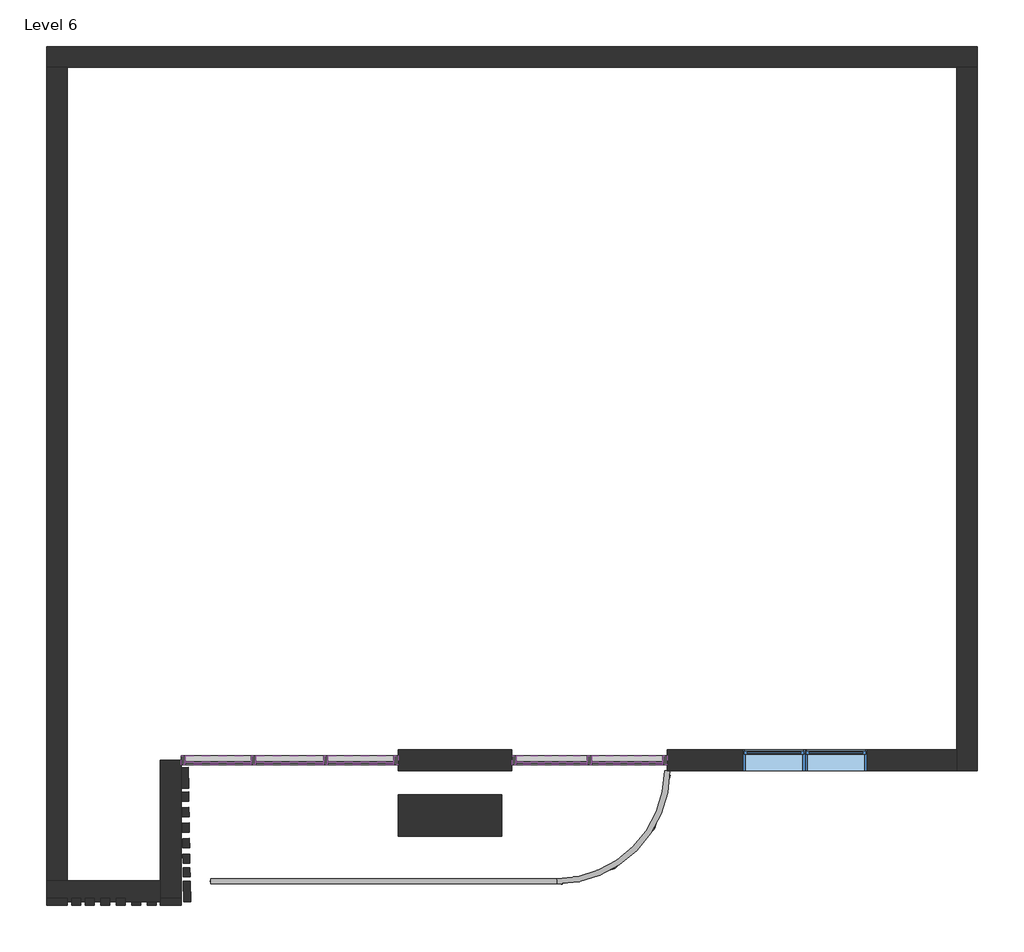
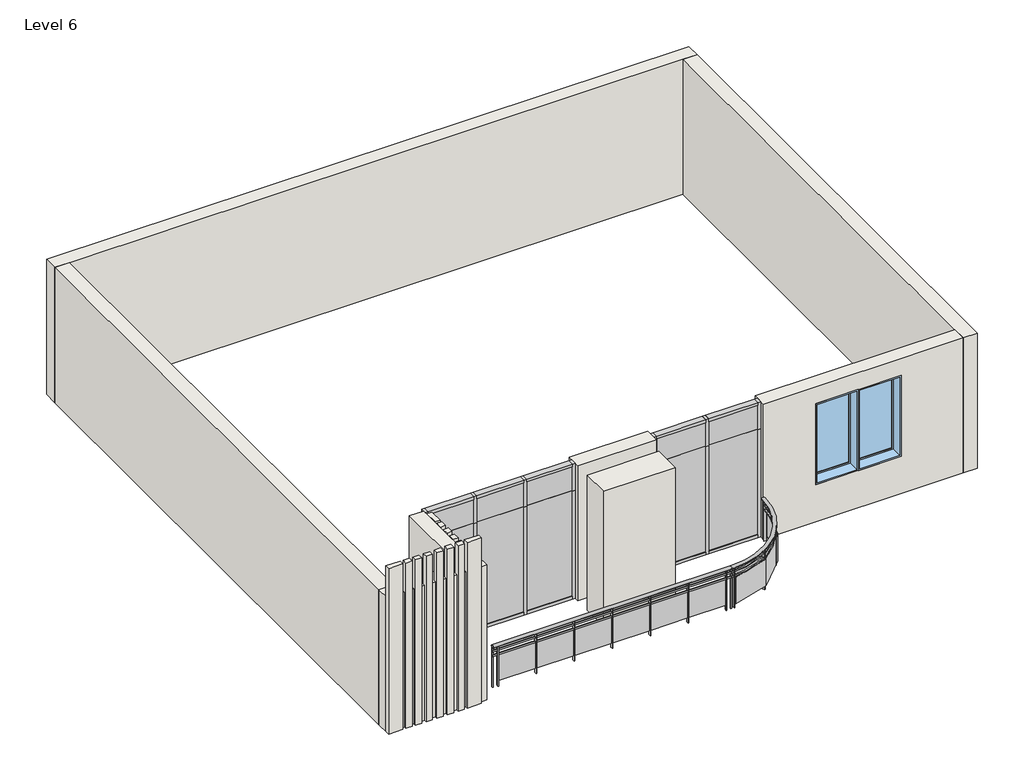
# One storey: 24 members, 24 walls, 10 plates, 2 windows, 1 railing.
"""IFC4 building model written with IfcOpenShell, lengths in millimetres."""

from ifc_helpers import new_model, si_unit, point, frame, origin, place, context, project, spatial, polyline, circle_curve, ellipse_curve, trimmed, outline, extrude, faceted_brep, transform, mapped, element, save
from ifc_brep_helpers import plane_surface, cylinder_surface, revolved_surface, extruded_surface, advanced_brep
from components import member_78934672, member_801a2072, member_cfcad22e, member_ee409385, member_47bfaf8a, member_f0fea5a5, member_6e77e263, system_panel_glazed_66ef8e2c, system_panel_glazed_30b75583, system_panel_glazed_387c9df4, system_panel_glazed_55a8196a, system_panel_glazed_9df4f396, system_panel_glazed_c1629c18, window_9a1f8bc2, window_c524ad49

model = new_model("IFC4")

# Units and contexts
model_context = context("Model", 3, world=origin())
ifc_project = project(units=[si_unit("LENGTHUNIT", "METRE", prefix="MILLI")], contexts=[model_context])

# Site, building, storey
site = spatial("IfcSite", under=ifc_project)
building = spatial("IfcBuilding", under=site)
storey = spatial("IfcBuildingStorey", under=building, Name="Level 6", Elevation=15240.0)

# Members
placement = place(None, origin())
member_shape = member_78934672(model_context)
element("IfcMember", 1, ObjectType="Rectangular Mullion : 2.5\" x 5\" rectangular", at=placement, inside=storey, context=model_context, shape_type="MappedRepresentation", body=[
    mapped(member_shape, transform((-10103.7104559, 977.728737, 14859.0), x_axis=(0.0, 0.0, -1.0), y_axis=(0.0, 1.0, 0.0), z_axis=(1.0, 0.0, 0.0))),
])
element("IfcMember", 2, ObjectType="Rectangular Mullion : 2.5\" x 5\" rectangular", at=placement, inside=storey, context=model_context, shape_type="MappedRepresentation", body=[
    mapped(member_shape, transform((-11214.9604559, 977.728737, 14859.0), x_axis=(0.0, 0.0, -1.0), y_axis=(0.0, 1.0, 0.0), z_axis=(1.0, 0.0, 0.0))),
])
element("IfcMember", 3, ObjectType="Rectangular Mullion : 2.5\" x 5\" rectangular", at=placement, inside=storey, context=model_context, shape_type="MappedRepresentation", body=[
    mapped(member_shape, transform((-12262.7104559, 977.728737, 17907.0), x_axis=(0.0, 0.0, 1.0), y_axis=(0.0, 1.0, 0.0), z_axis=(-1.0, 0.0, 0.0))),
])
element("IfcMember", 4, ObjectType="Rectangular Mullion : 2.5\" x 5\" rectangular", at=placement, inside=storey, context=model_context, shape_type="MappedRepresentation", body=[
    mapped(member_shape, transform((-11151.4604559, 977.728737, 17907.0), x_axis=(0.0, 0.0, 1.0), y_axis=(0.0, 1.0, 0.0), z_axis=(-1.0, 0.0, 0.0))),
])
member_2_shape = member_801a2072(model_context)
element("IfcMember", 5, ObjectType="Rectangular Mullion : 2.5\" x 5\" rectangular", at=placement, inside=storey, context=model_context, shape_type="MappedRepresentation", body=[
    mapped(member_2_shape, transform((-17139.5104559, 977.728737, 17907.0), x_axis=(0.0, 0.0, 1.0), y_axis=(0.0, 1.0, 0.0), z_axis=(-1.0, 0.0, 0.0))),
])
element("IfcMember", 6, ObjectType="Rectangular Mullion : 2.5\" x 5\" rectangular", at=placement, inside=storey, context=model_context, shape_type="MappedRepresentation", body=[
    mapped(member_2_shape, transform((-15037.6604559, 977.728737, 17907.0), x_axis=(0.0, 0.0, 1.0), y_axis=(0.0, 1.0, 0.0), z_axis=(-1.0, 0.0, 0.0))),
])
element("IfcMember", 7, ObjectType="Rectangular Mullion : 2.5\" x 5\" rectangular", at=placement, inside=storey, context=model_context, shape_type="MappedRepresentation", body=[
    mapped(member_2_shape, transform((-14066.1104559, 977.728737, 14859.0), x_axis=(0.0, 0.0, -1.0), y_axis=(0.0, 1.0, 0.0), z_axis=(1.0, 0.0, 0.0))),
])
element("IfcMember", 8, ObjectType="Rectangular Mullion : 2.5\" x 5\" rectangular", at=placement, inside=storey, context=model_context, shape_type="MappedRepresentation", body=[
    mapped(member_2_shape, transform((-16167.9604559, 977.728737, 14859.0), x_axis=(0.0, 0.0, -1.0), y_axis=(0.0, 1.0, 0.0), z_axis=(1.0, 0.0, 0.0))),
])
member_3_shape = member_cfcad22e(model_context)
element("IfcMember", 9, ObjectType="Rectangular Mullion : 2.5\" x 5\" rectangular", at=placement, inside=storey, context=model_context, shape_type="MappedRepresentation", body=[
    mapped(member_3_shape, transform((-15101.1604559, 977.728737, 14859.0), x_axis=(0.0, 0.0, -1.0), y_axis=(0.0, 1.0, 0.0), z_axis=(1.0, 0.0, 0.0))),
])
element("IfcMember", 10, ObjectType="Rectangular Mullion : 2.5\" x 5\" rectangular", at=placement, inside=storey, context=model_context, shape_type="MappedRepresentation", body=[
    mapped(member_3_shape, transform((-16104.4604559, 977.728737, 17907.0), x_axis=(0.0, 0.0, 1.0), y_axis=(0.0, 1.0, 0.0), z_axis=(-1.0, 0.0, 0.0))),
])
member_4_shape = member_ee409385(model_context)
element("IfcMember", 11, ObjectType="Rectangular Mullion : 2.5\" x 5\" rectangular", at=placement, inside=storey, context=model_context, shape_type="MappedRepresentation", body=[
    mapped(member_4_shape, transform((-12326.2104559, 977.728737, 14859.0), x_axis=(-1.0, 0.0, 0.0), y_axis=(0.0, 1.0, 0.0), z_axis=(0.0, 0.0, -1.0))),
])
element("IfcMember", 12, ObjectType="Rectangular Mullion : 2.5\" x 5\" rectangular", at=placement, inside=storey, context=model_context, shape_type="MappedRepresentation", body=[
    mapped(member_4_shape, transform((-17203.0104559, 977.728737, 14859.0), x_axis=(-1.0, 0.0, 0.0), y_axis=(0.0, 1.0, 0.0), z_axis=(0.0, 0.0, -1.0))),
])
member_5_shape = member_47bfaf8a(model_context)
element("IfcMember", 13, ObjectType="Rectangular Mullion : 2.5\" x 5\" rectangular", at=placement, inside=storey, context=model_context, shape_type="MappedRepresentation", body=[
    mapped(member_5_shape, transform((-12326.2104559, 977.728737, 17297.4), x_axis=(-1.0, 0.0, 0.0), y_axis=(0.0, 1.0, 0.0), z_axis=(0.0, 0.0, -1.0))),
])
element("IfcMember", 14, ObjectType="Rectangular Mullion : 2.5\" x 5\" rectangular", at=placement, inside=storey, context=model_context, shape_type="MappedRepresentation", body=[
    mapped(member_5_shape, transform((-17203.0104559, 977.728737, 17297.4), x_axis=(-1.0, 0.0, 0.0), y_axis=(0.0, 1.0, 0.0), z_axis=(0.0, 0.0, -1.0))),
])
member_6_shape = member_f0fea5a5(model_context)
element("IfcMember", 15, ObjectType="Rectangular Mullion : 2.5\" x 5\" rectangular", at=placement, inside=storey, context=model_context, shape_type="MappedRepresentation", body=[
    mapped(member_6_shape, transform((-11183.2104559, 977.728737, 14859.0), x_axis=(-1.0, 0.0, 0.0), y_axis=(0.0, 1.0, 0.0), z_axis=(0.0, 0.0, -1.0))),
])
element("IfcMember", 16, ObjectType="Rectangular Mullion : 2.5\" x 5\" rectangular", at=placement, inside=storey, context=model_context, shape_type="MappedRepresentation", body=[
    mapped(member_6_shape, transform((-15069.4104559, 977.728737, 14859.0), x_axis=(-1.0, 0.0, 0.0), y_axis=(0.0, 1.0, 0.0), z_axis=(0.0, 0.0, -1.0))),
])
element("IfcMember", 17, ObjectType="Rectangular Mullion : 2.5\" x 5\" rectangular", at=placement, inside=storey, context=model_context, shape_type="MappedRepresentation", body=[
    mapped(member_6_shape, transform((-16136.2104559, 977.728737, 14859.0), x_axis=(-1.0, 0.0, 0.0), y_axis=(0.0, 1.0, 0.0), z_axis=(0.0, 0.0, -1.0))),
])
member_7_shape = member_6e77e263(model_context)
element("IfcMember", 18, ObjectType="Rectangular Mullion : 2.5\" x 5\" rectangular", at=placement, inside=storey, context=model_context, shape_type="MappedRepresentation", body=[
    mapped(member_7_shape, transform((-11183.2104559, 977.728737, 17297.4), x_axis=(-1.0, 0.0, 0.0), y_axis=(0.0, 1.0, 0.0), z_axis=(0.0, 0.0, -1.0))),
])
element("IfcMember", 19, ObjectType="Rectangular Mullion : 2.5\" x 5\" rectangular", at=placement, inside=storey, context=model_context, shape_type="MappedRepresentation", body=[
    mapped(member_7_shape, transform((-15069.4104559, 977.728737, 17297.4), x_axis=(-1.0, 0.0, 0.0), y_axis=(0.0, 1.0, 0.0), z_axis=(0.0, 0.0, -1.0))),
])
element("IfcMember", 20, ObjectType="Rectangular Mullion : 2.5\" x 5\" rectangular", at=placement, inside=storey, context=model_context, shape_type="MappedRepresentation", body=[
    mapped(member_7_shape, transform((-16136.2104559, 977.728737, 17297.4), x_axis=(-1.0, 0.0, 0.0), y_axis=(0.0, 1.0, 0.0), z_axis=(0.0, 0.0, -1.0))),
])
element("IfcMember", 21, ObjectType="Rectangular Mullion : 2.5\" x 5\" rectangular", at=placement, inside=storey, context=model_context, shape_type="MappedRepresentation", body=[
    mapped(member_5_shape, transform((-10040.2104559, 977.728737, 17907.0), x_axis=(1.0, 0.0, 0.0), y_axis=(0.0, 1.0, 0.0), z_axis=(0.0, 0.0, 1.0))),
])
element("IfcMember", 22, ObjectType="Rectangular Mullion : 2.5\" x 5\" rectangular", at=placement, inside=storey, context=model_context, shape_type="MappedRepresentation", body=[
    mapped(member_5_shape, transform((-14002.6104559, 977.728737, 17907.0), x_axis=(1.0, 0.0, 0.0), y_axis=(0.0, 1.0, 0.0), z_axis=(0.0, 0.0, 1.0))),
])
element("IfcMember", 23, ObjectType="Rectangular Mullion : 2.5\" x 5\" rectangular", at=placement, inside=storey, context=model_context, shape_type="MappedRepresentation", body=[
    mapped(member_4_shape, transform((-10040.2104559, 977.728737, 17297.4), x_axis=(1.0, 0.0, 0.0), y_axis=(0.0, 1.0, 0.0), z_axis=(0.0, 0.0, 1.0))),
])
element("IfcMember", 24, ObjectType="Rectangular Mullion : 2.5\" x 5\" rectangular", at=placement, inside=storey, context=model_context, shape_type="MappedRepresentation", body=[
    mapped(member_4_shape, transform((-14002.6104559, 977.728737, 17297.4), x_axis=(1.0, 0.0, 0.0), y_axis=(0.0, 1.0, 0.0), z_axis=(0.0, 0.0, 1.0))),
])

# Plates
system_panel_glazed_shape = system_panel_glazed_66ef8e2c(model_context)
element("IfcPlate", 25, ObjectType="System Panel : Glazed", at=placement, inside=storey, context=model_context, shape_type="MappedRepresentation", body=[
    mapped(system_panel_glazed_shape, transform((-10627.5854559, 977.728737, 14922.5), x_axis=(-1.0, 0.0, 0.0), y_axis=(0.0, -1.0, 0.0), z_axis=(0.0, 0.0, 1.0))),
])
element("IfcPlate", 26, ObjectType="System Panel : Glazed", at=placement, inside=storey, context=model_context, shape_type="MappedRepresentation", body=[
    mapped(system_panel_glazed_shape, transform((-11738.8354559, 977.728737, 14922.5), x_axis=(-1.0, 0.0, 0.0), y_axis=(0.0, -1.0, 0.0), z_axis=(0.0, 0.0, 1.0))),
])
system_panel_glazed_2_shape = system_panel_glazed_30b75583(model_context)
element("IfcPlate", 27, ObjectType="System Panel : Glazed", at=placement, inside=storey, context=model_context, shape_type="MappedRepresentation", body=[
    mapped(system_panel_glazed_2_shape, transform((-10627.5854559, 977.728737, 17297.4), x_axis=(-1.0, 0.0, 0.0), y_axis=(0.0, -1.0, 0.0), z_axis=(0.0, 0.0, 1.0))),
])
element("IfcPlate", 28, ObjectType="System Panel : Glazed", at=placement, inside=storey, context=model_context, shape_type="MappedRepresentation", body=[
    mapped(system_panel_glazed_2_shape, transform((-11738.8354559, 977.728737, 17297.4), x_axis=(-1.0, 0.0, 0.0), y_axis=(0.0, -1.0, 0.0), z_axis=(0.0, 0.0, 1.0))),
])
system_panel_glazed_3_shape = system_panel_glazed_387c9df4(model_context)
element("IfcPlate", 29, ObjectType="System Panel : Glazed", at=placement, inside=storey, context=model_context, shape_type="MappedRepresentation", body=[
    mapped(system_panel_glazed_3_shape, transform((-14551.8854559, 977.728737, 14922.5), x_axis=(-1.0, 0.0, 0.0), y_axis=(0.0, -1.0, 0.0), z_axis=(0.0, 0.0, 1.0))),
])
element("IfcPlate", 30, ObjectType="System Panel : Glazed", at=placement, inside=storey, context=model_context, shape_type="MappedRepresentation", body=[
    mapped(system_panel_glazed_3_shape, transform((-16653.7354559, 977.728737, 14922.5), x_axis=(-1.0, 0.0, 0.0), y_axis=(0.0, -1.0, 0.0), z_axis=(0.0, 0.0, 1.0))),
])
system_panel_glazed_4_shape = system_panel_glazed_55a8196a(model_context)
element("IfcPlate", 31, ObjectType="System Panel : Glazed", at=placement, inside=storey, context=model_context, shape_type="MappedRepresentation", body=[
    mapped(system_panel_glazed_4_shape, transform((-14551.8854559, 977.728737, 17297.4), x_axis=(-1.0, 0.0, 0.0), y_axis=(0.0, -1.0, 0.0), z_axis=(0.0, 0.0, 1.0))),
])
element("IfcPlate", 32, ObjectType="System Panel : Glazed", at=placement, inside=storey, context=model_context, shape_type="MappedRepresentation", body=[
    mapped(system_panel_glazed_4_shape, transform((-16653.7354559, 977.728737, 17297.4), x_axis=(-1.0, 0.0, 0.0), y_axis=(0.0, -1.0, 0.0), z_axis=(0.0, 0.0, 1.0))),
])
system_panel_glazed_5_shape = system_panel_glazed_9df4f396(model_context)
element("IfcPlate", 33, ObjectType="System Panel : Glazed", at=placement, inside=storey, context=model_context, shape_type="MappedRepresentation", body=[
    mapped(system_panel_glazed_5_shape, transform((-15602.8104559, 977.728737, 14922.5), x_axis=(-1.0, 0.0, 0.0), y_axis=(0.0, -1.0, 0.0), z_axis=(0.0, 0.0, 1.0))),
])
system_panel_glazed_6_shape = system_panel_glazed_c1629c18(model_context)
element("IfcPlate", 34, ObjectType="System Panel : Glazed", at=placement, inside=storey, context=model_context, shape_type="MappedRepresentation", body=[
    mapped(system_panel_glazed_6_shape, transform((-15602.8104559, 977.728737, 17297.4), x_axis=(-1.0, 0.0, 0.0), y_axis=(0.0, -1.0, 0.0), z_axis=(0.0, 0.0, 1.0))),
])

# Railing
element("IfcRailing", 35, ObjectType="Glass Panel - Bottom Fill", at=placement, inside=storey, context=model_context, shape_type="SolidModel", body=[
    advanced_brep(
    [(-16762.7787181, -765.7171954, 15773.4), (-16762.7787181, -841.9171954, 15773.4), (-11669.3563882, -765.7171954, 15773.4), (-11669.3563882, -841.9171954, 15773.4), (-10002.1104559, 825.328737, 15773.4), (-10078.3104559, 825.328737, 15773.4)],
    [
        (0, 1, ellipse_curve(frame((-16762.7787181, -803.8171954, 15773.4), z_axis=(-1.0, 0.0, 0.0), x_axis=(0.0, -1.0, 0.0)), 38.1, 28.575)),
        (1, 0, ellipse_curve(frame((-16762.7787181, -803.8171954, 15773.4), z_axis=(-1.0, 0.0, 0.0), x_axis=(0.0, -1.0, 0.0)), 38.1, 28.575)),
        (0, 2),
        (2, 3, ellipse_curve(frame((-11669.3563882, -803.8171954, 15773.4), z_axis=(-1.0, 0.0, 0.0), x_axis=(0.0, -1.0, 0.0)), 38.1, 28.575)),
        (3, 1),
        (3, 2, ellipse_curve(frame((-11669.3563882, -803.8171954, 15773.4), z_axis=(-1.0, 0.0, 0.0), x_axis=(0.0, -1.0, 0.0)), 38.1, 28.575)),
        (4, 3, circle_curve(frame((-11669.3563882, 825.328737, 15773.4), z_axis=(0.0, 0.0, -1.0), x_axis=(0.0, -1.0, 0.0)), 1667.2459324)),
        (2, 5, circle_curve(frame((-11669.3563882, 825.328737, 15773.4), z_axis=(0.0, 0.0, 1.0), x_axis=(0.0, -1.0, 0.0)), 1591.0459324)),
        (5, 4, ellipse_curve(frame((-10040.2104559, 825.328737, 15773.4), z_axis=(0.0, -1.0, 0.0), x_axis=(1.0, 0.0, 0.0)), 38.1, 28.575)),
        (4, 5, ellipse_curve(frame((-10040.2104559, 825.328737, 15773.4), z_axis=(0.0, -1.0, 0.0), x_axis=(1.0, 0.0, 0.0)), 38.1, 28.575)),
    ],
    [
        plane_surface(frame((-16762.7787181, -803.8171954, 15773.4), z_axis=(-1.0, 0.0, 0.0), x_axis=(0.0, 1.0, 0.0))),
        extruded_surface(trimmed(ellipse_curve(frame((-11669.3563882, -803.8171954, 15773.4), z_axis=(-1.0, 0.0, 0.0), x_axis=(0.0, -1.0, 0.0)), 38.1, 28.575), [point((-11669.3563882, -765.7171954, 15773.4))], [point((-11669.3563882, -841.9171954, 15773.4))], True, "CARTESIAN"), (-5093.422329899999, 0.0, 0.0), 5093.422329899999),
        extruded_surface(trimmed(ellipse_curve(frame((-11669.3563882, -803.8171954, 15773.4), z_axis=(-1.0, 0.0, 0.0), x_axis=(0.0, -1.0, 0.0)), 38.1, 28.575), [point((-11669.3563882, -841.9171954, 15773.4))], [point((-11669.3563882, -765.7171954, 15773.4))], True, "CARTESIAN"), (-5093.422329899999, 0.0, 0.0), 5093.422329899999),
        revolved_surface(trimmed(ellipse_curve(frame((-11669.3563882, -803.8171954, 15773.4), z_axis=(-1.0, 0.0, 0.0), x_axis=(0.0, -1.0, 0.0)), 38.1, 28.575), [point((-11669.3563882, -765.7171954, 15773.4))], [point((-11669.3563882, -841.9171954, 15773.4))], True, "CARTESIAN"), (-11669.3563882, 825.328737, 15773.4), (0.0, 0.0, 1.0)),
        revolved_surface(trimmed(ellipse_curve(frame((-11669.3563882, -803.8171954, 15773.4), z_axis=(-1.0, 0.0, 0.0), x_axis=(0.0, -1.0, 0.0)), 38.1, 28.575), [point((-11669.3563882, -841.9171954, 15773.4))], [point((-11669.3563882, -765.7171954, 15773.4))], True, "CARTESIAN"), (-11669.3563882, 825.328737, 15773.4), (0.0, 0.0, 1.0)),
        plane_surface(frame((-10040.2104559, 825.328737, 15773.4), z_axis=(0.0, 1.0, 0.0), x_axis=(0.0, 0.0, 1.0))),
    ],
    [
        (0, [[1, 2]]),
        (1, [[-1, 3, 4, 5]]),
        (2, [[-2, -5, 6, -3]]),
        (3, [[7, -4, 8, 9]]),
        (4, [[-8, -6, -7, 10]]),
        (5, [[-10, -9]]),
    ],
),
    advanced_brep(
    [(-16762.7787181, -816.5171954, 15684.5), (-16762.7787181, -791.1171954, 15684.5), (-16762.7787181, -791.1171954, 15659.1), (-16762.7787181, -816.5171954, 15659.1), (-11669.3563882, -816.5171954, 15684.5), (-11669.3563882, -791.1171954, 15684.5), (-11669.3563882, -791.1171954, 15659.1), (-11669.3563882, -816.5171954, 15659.1), (-10052.9104559, 825.328737, 15684.5), (-10027.5104559, 825.328737, 15684.5), (-10052.9104559, 825.328737, 15659.1), (-10027.5104559, 825.328737, 15659.1)],
    [
        (0, 1),
        (1, 2),
        (2, 3),
        (3, 0),
        (0, 4),
        (4, 5),
        (5, 1),
        (5, 6),
        (6, 2),
        (6, 7),
        (7, 3),
        (7, 4),
        (8, 5, circle_curve(frame((-11669.3563882, 825.328737, 15684.5), z_axis=(0.0, 0.0, -1.0), x_axis=(0.0, -1.0, 0.0)), 1616.4459324)),
        (4, 9, circle_curve(frame((-11669.3563882, 825.328737, 15684.5), z_axis=(0.0, 0.0, 1.0), x_axis=(0.0, -1.0, 0.0)), 1641.8459324)),
        (9, 8),
        (10, 6, circle_curve(frame((-11669.3563882, 825.328737, 15659.1), z_axis=(0.0, 0.0, -1.0), x_axis=(0.0, -1.0, 0.0)), 1616.4459324)),
        (8, 10),
        (11, 7, circle_curve(frame((-11669.3563882, 825.328737, 15659.1), z_axis=(0.0, 0.0, -1.0), x_axis=(0.0, -1.0, 0.0)), 1641.8459324)),
        (10, 11),
        (11, 9),
    ],
    [
        plane_surface(frame((-16762.7787181, -803.8171954, 15671.8), z_axis=(-1.0, 0.0, 0.0), x_axis=(0.0, 1.0, 0.0))),
        plane_surface(frame((-16762.7787181, -816.5171954, 15684.5), z_axis=(0.0, 0.0, 1.0), x_axis=(1.0, 0.0, 0.0))),
        plane_surface(frame((-16762.7787181, -791.1171954, 15684.5), z_axis=(0.0, 1.0, 0.0), x_axis=(1.0, 0.0, 0.0))),
        plane_surface(frame((-16762.7787181, -791.1171954, 15659.1), z_axis=(0.0, 0.0, -1.0), x_axis=(1.0, 0.0, 0.0))),
        plane_surface(frame((-16762.7787181, -816.5171954, 15659.1), z_axis=(0.0, -1.0, 0.0), x_axis=(1.0, 0.0, 0.0))),
        plane_surface(frame((-11669.3563882, 825.328737, 15684.5), z_axis=(0.0, 0.0, 1.0), x_axis=(0.0, -1.0, 0.0))),
        revolved_surface(polyline([(-11669.3563882, -791.1171953999999, 15684.5), (-11669.3563882, -791.1171953999999, 15659.1)]), (-11669.3563882, 825.328737, 15671.8), (0.0, 0.0, 1.0)),
        plane_surface(frame((-11669.3563882, 825.328737, 15659.1), z_axis=(0.0, 0.0, -1.0), x_axis=(0.0, -1.0, 0.0))),
        cylinder_surface(frame((-11669.3563882, 825.328737, 15671.8), z_axis=(0.0, 0.0, 1.0), x_axis=(0.0, -1.0, 0.0)), 1641.8459324),
        plane_surface(frame((-10040.2104559, 825.328737, 15671.8), z_axis=(0.0, 1.0, 0.0), x_axis=(0.0, 0.0, 1.0))),
    ],
    [
        (0, [[1, 2, 3, 4]]),
        (1, [[-1, 5, 6, 7]]),
        (2, [[-2, -7, 8, 9]]),
        (3, [[-3, -9, 10, 11]]),
        (4, [[-4, -11, 12, -5]]),
        (5, [[13, -6, 14, 15]]),
        (6, [[16, -8, -13, 17]]),
        (7, [[18, -10, -16, 19]]),
        (8, [[-14, -12, -18, 20]]),
        (9, [[-20, -19, -17, -15]]),
    ],
),
    advanced_brep(
    [(-16762.7787181, -816.5171954, 15582.9), (-16762.7787181, -791.1171954, 15582.9), (-16762.7787181, -791.1171954, 15557.5), (-16762.7787181, -816.5171954, 15557.5), (-11669.3563882, -816.5171954, 15582.9), (-11669.3563882, -791.1171954, 15582.9), (-11669.3563882, -791.1171954, 15557.5), (-11669.3563882, -816.5171954, 15557.5), (-10052.9104559, 825.328737, 15582.9), (-10027.5104559, 825.328737, 15582.9), (-10052.9104559, 825.328737, 15557.5), (-10027.5104559, 825.328737, 15557.5)],
    [
        (0, 1),
        (1, 2),
        (2, 3),
        (3, 0),
        (0, 4),
        (4, 5),
        (5, 1),
        (5, 6),
        (6, 2),
        (6, 7),
        (7, 3),
        (7, 4),
        (8, 5, circle_curve(frame((-11669.3563882, 825.328737, 15582.9), z_axis=(0.0, 0.0, -1.0), x_axis=(0.0, -1.0, 0.0)), 1616.4459324)),
        (4, 9, circle_curve(frame((-11669.3563882, 825.328737, 15582.9), z_axis=(0.0, 0.0, 1.0), x_axis=(0.0, -1.0, 0.0)), 1641.8459324)),
        (9, 8),
        (10, 6, circle_curve(frame((-11669.3563882, 825.328737, 15557.5), z_axis=(0.0, 0.0, -1.0), x_axis=(0.0, -1.0, 0.0)), 1616.4459324)),
        (8, 10),
        (11, 7, circle_curve(frame((-11669.3563882, 825.328737, 15557.5), z_axis=(0.0, 0.0, -1.0), x_axis=(0.0, -1.0, 0.0)), 1641.8459324)),
        (10, 11),
        (11, 9),
    ],
    [
        plane_surface(frame((-16762.7787181, -803.8171954, 15570.2), z_axis=(-1.0, 0.0, 0.0), x_axis=(0.0, 1.0, 0.0))),
        plane_surface(frame((-16762.7787181, -816.5171954, 15582.9), z_axis=(0.0, 0.0, 1.0), x_axis=(1.0, 0.0, 0.0))),
        plane_surface(frame((-16762.7787181, -791.1171954, 15582.9), z_axis=(0.0, 1.0, 0.0), x_axis=(1.0, 0.0, 0.0))),
        plane_surface(frame((-16762.7787181, -791.1171954, 15557.5), z_axis=(0.0, 0.0, -1.0), x_axis=(1.0, 0.0, 0.0))),
        plane_surface(frame((-16762.7787181, -816.5171954, 15557.5), z_axis=(0.0, -1.0, 0.0), x_axis=(1.0, 0.0, 0.0))),
        plane_surface(frame((-11669.3563882, 825.328737, 15582.9), z_axis=(0.0, 0.0, 1.0), x_axis=(0.0, -1.0, 0.0))),
        revolved_surface(polyline([(-11669.3563882, -791.1171953999999, 15582.9), (-11669.3563882, -791.1171953999999, 15557.5)]), (-11669.3563882, 825.328737, 15570.2), (0.0, 0.0, 1.0)),
        plane_surface(frame((-11669.3563882, 825.328737, 15557.5), z_axis=(0.0, 0.0, -1.0), x_axis=(0.0, -1.0, 0.0))),
        cylinder_surface(frame((-11669.3563882, 825.328737, 15570.2), z_axis=(0.0, 0.0, 1.0), x_axis=(0.0, -1.0, 0.0)), 1641.8459324),
        plane_surface(frame((-10040.2104559, 825.328737, 15570.2), z_axis=(0.0, 1.0, 0.0), x_axis=(0.0, 0.0, 1.0))),
    ],
    [
        (0, [[1, 2, 3, 4]]),
        (1, [[-1, 5, 6, 7]]),
        (2, [[-2, -7, 8, 9]]),
        (3, [[-3, -9, 10, 11]]),
        (4, [[-4, -11, 12, -5]]),
        (5, [[13, -6, 14, 15]]),
        (6, [[16, -8, -13, 17]]),
        (7, [[18, -10, -16, 19]]),
        (8, [[-14, -12, -18, 20]]),
        (9, [[-20, -19, -17, -15]]),
    ],
),
    extrude(outline(polyline([(-10016.1798264, 757.7282919), (-10066.9450003, 759.6090156), (-10066.4748193, 772.3003091), (-10015.7096455, 770.4195853), (-10016.1798264, 757.7282919)])), frame((0.0, 0.0, 14859.0), z_axis=(0.0, 0.0, 1.0), x_axis=(1.0, 0.0, 0.0)), (0.0, 0.0, 1.0), 885.6788223),
    extrude(outline(polyline([(-10227.7208829, -23.0307141), (-9998.0369146, 756.6417265), (-9991.9457237, 754.8473205), (-10221.629692, -24.8251201), (-10227.7208829, -23.0307141)])), frame((0.0, 0.0, 14960.6), z_axis=(0.0, 0.0, 1.0), x_axis=(1.0, 0.0, 0.0)), (0.0, 0.0, 1.0), 596.9),
    extrude(outline(polyline([(-10250.0405804, -25.0271899), (-10293.7178017, 0.9139036), (-10287.2325284, 11.8332089), (-10243.555307, -14.1078846), (-10250.0405804, -25.0271899)])), frame((0.0, 0.0, 14859.0), z_axis=(0.0, 0.0, 1.0), x_axis=(1.0, 0.0, 0.0)), (0.0, 0.0, 1.0), 885.6788223),
    extrude(outline(polyline([(-10809.3655016, -609.3985414), (-10234.6291099, -34.6621497), (-10230.1389818, -39.1522777), (-10804.8753736, -613.8886695), (-10809.3655016, -609.3985414)])), frame((0.0, 0.0, 14960.6), z_axis=(0.0, 0.0, 1.0), x_axis=(1.0, 0.0, 0.0)), (0.0, 0.0, 1.0), 596.9),
    extrude(outline(polyline([(-10829.9197667, -600.4723443), (-10855.8608602, -556.7951229), (-10844.9415549, -550.3098495), (-10819.0004614, -593.9870709), (-10829.9197667, -600.4723443)])), frame((0.0, 0.0, 14859.0), z_axis=(0.0, 0.0, 1.0), x_axis=(1.0, 0.0, 0.0)), (0.0, 0.0, 1.0), 885.6788223),
    extrude(outline(polyline([(-11600.6693778, -845.9907367), (-10820.9969372, -616.3067684), (-10819.2025312, -622.3979593), (-11598.8749718, -852.0819276), (-11600.6693778, -845.9907367)])), frame((0.0, 0.0, 14960.6), z_axis=(0.0, 0.0, 1.0), x_axis=(1.0, 0.0, 0.0)), (0.0, 0.0, 1.0), 596.9),
    extrude(outline(polyline([(-11614.4472366, -828.3180058), (-11616.3279603, -777.552832), (-11603.6366669, -777.082651), (-11601.7559432, -827.8478249), (-11614.4472366, -828.3180058)])), frame((0.0, 0.0, 14859.0), z_axis=(0.0, 0.0, 1.0), x_axis=(1.0, 0.0, 0.0)), (0.0, 0.0, 1.0), 885.6788223),
    extrude(outline(polyline([(-11784.0175532, -829.2171954), (-11784.0175532, -778.4171954), (-11771.3175532, -778.4171954), (-11771.3175532, -829.2171954), (-11784.0175532, -829.2171954)])), frame((0.0, 0.0, 14859.0), z_axis=(0.0, 0.0, 1.0), x_axis=(1.0, 0.0, 0.0)), (0.0, 0.0, 1.0), 885.6788223),
    extrude(outline(polyline([(-12590.4675532, -797.2820384), (-11777.6675532, -797.2820384), (-11777.6675532, -803.6320384), (-12590.4675532, -803.6320384), (-12590.4675532, -797.2820384)])), frame((0.0, 0.0, 14960.6), z_axis=(0.0, 0.0, 1.0), x_axis=(1.0, 0.0, 0.0)), (0.0, 0.0, 1.0), 596.9),
    extrude(outline(polyline([(-12596.8175532, -829.2171954), (-12596.8175532, -778.4171954), (-12584.1175532, -778.4171954), (-12584.1175532, -829.2171954), (-12596.8175532, -829.2171954)])), frame((0.0, 0.0, 14859.0), z_axis=(0.0, 0.0, 1.0), x_axis=(1.0, 0.0, 0.0)), (0.0, 0.0, 1.0), 885.6788223),
    extrude(outline(polyline([(-13403.2675532, -797.2820384), (-12590.4675532, -797.2820384), (-12590.4675532, -803.6320384), (-13403.2675532, -803.6320384), (-13403.2675532, -797.2820384)])), frame((0.0, 0.0, 14960.6), z_axis=(0.0, 0.0, 1.0), x_axis=(1.0, 0.0, 0.0)), (0.0, 0.0, 1.0), 596.9),
    extrude(outline(polyline([(-13409.6175532, -829.2171954), (-13409.6175532, -778.4171954), (-13396.9175532, -778.4171954), (-13396.9175532, -829.2171954), (-13409.6175532, -829.2171954)])), frame((0.0, 0.0, 14859.0), z_axis=(0.0, 0.0, 1.0), x_axis=(1.0, 0.0, 0.0)), (0.0, 0.0, 1.0), 885.6788223),
    extrude(outline(polyline([(-14216.0675532, -797.2820384), (-13403.2675532, -797.2820384), (-13403.2675532, -803.6320384), (-14216.0675532, -803.6320384), (-14216.0675532, -797.2820384)])), frame((0.0, 0.0, 14960.6), z_axis=(0.0, 0.0, 1.0), x_axis=(1.0, 0.0, 0.0)), (0.0, 0.0, 1.0), 596.9),
    extrude(outline(polyline([(-14222.4175532, -829.2171954), (-14222.4175532, -778.4171954), (-14209.7175532, -778.4171954), (-14209.7175532, -829.2171954), (-14222.4175532, -829.2171954)])), frame((0.0, 0.0, 14859.0), z_axis=(0.0, 0.0, 1.0), x_axis=(1.0, 0.0, 0.0)), (0.0, 0.0, 1.0), 885.6788223),
    extrude(outline(polyline([(-15028.8675532, -797.2820384), (-14216.0675532, -797.2820384), (-14216.0675532, -803.6320384), (-15028.8675532, -803.6320384), (-15028.8675532, -797.2820384)])), frame((0.0, 0.0, 14960.6), z_axis=(0.0, 0.0, 1.0), x_axis=(1.0, 0.0, 0.0)), (0.0, 0.0, 1.0), 596.9),
    extrude(outline(polyline([(-15035.2175532, -829.2171954), (-15035.2175532, -778.4171954), (-15022.5175532, -778.4171954), (-15022.5175532, -829.2171954), (-15035.2175532, -829.2171954)])), frame((0.0, 0.0, 14859.0), z_axis=(0.0, 0.0, 1.0), x_axis=(1.0, 0.0, 0.0)), (0.0, 0.0, 1.0), 885.6788223),
    extrude(outline(polyline([(-15841.6675532, -797.2820384), (-15028.8675532, -797.2820384), (-15028.8675532, -803.6320384), (-15841.6675532, -803.6320384), (-15841.6675532, -797.2820384)])), frame((0.0, 0.0, 14960.6), z_axis=(0.0, 0.0, 1.0), x_axis=(1.0, 0.0, 0.0)), (0.0, 0.0, 1.0), 596.9),
    extrude(outline(polyline([(-15848.0175532, -829.2171954), (-15848.0175532, -778.4171954), (-15835.3175532, -778.4171954), (-15835.3175532, -829.2171954), (-15848.0175532, -829.2171954)])), frame((0.0, 0.0, 14859.0), z_axis=(0.0, 0.0, 1.0), x_axis=(1.0, 0.0, 0.0)), (0.0, 0.0, 1.0), 885.6788223),
    extrude(outline(polyline([(-16654.4675532, -797.2820384), (-15841.6675532, -797.2820384), (-15841.6675532, -803.6320384), (-16654.4675532, -803.6320384), (-16654.4675532, -797.2820384)])), frame((0.0, 0.0, 14960.6), z_axis=(0.0, 0.0, 1.0), x_axis=(1.0, 0.0, 0.0)), (0.0, 0.0, 1.0), 596.9),
    extrude(outline(polyline([(-16660.8175532, -829.2171954), (-16660.8175532, -778.4171954), (-16648.1175532, -778.4171954), (-16648.1175532, -829.2171954), (-16660.8175532, -829.2171954)])), frame((0.0, 0.0, 14859.0), z_axis=(0.0, 0.0, 1.0), x_axis=(1.0, 0.0, 0.0)), (0.0, 0.0, 1.0), 885.6788223),
    extrude(outline(polyline([(-11678.8813882, -813.3421954), (-11678.8813882, -794.2921954), (-11659.8313882, -794.2921954), (-11659.8313882, -813.3421954), (-11678.8813882, -813.3421954)])), frame((0.0, 0.0, 14859.0), z_axis=(0.0, 0.0, 1.0), x_axis=(1.0, 0.0, 0.0)), (0.0, 0.0, 1.0), 885.6788223),
    extrude(outline(polyline([(-10030.7071308, 812.610194), (-10049.7570946, 812.6473201), (-10049.7199686, 831.6972839), (-10030.6700048, 831.6601579), (-10030.7071308, 812.610194)])), frame((0.0, 0.0, 14859.0), z_axis=(0.0, 0.0, 1.0), x_axis=(1.0, 0.0, 0.0)), (0.0, 0.0, 1.0), 885.6788223),
    extrude(outline(polyline([(-16769.1287181, -813.3421954), (-16769.1287181, -794.2921954), (-16750.0787181, -794.2921954), (-16750.0787181, -813.3421954), (-16769.1287181, -813.3421954)])), frame((0.0, 0.0, 14859.0), z_axis=(0.0, 0.0, 1.0), x_axis=(1.0, 0.0, 0.0)), (0.0, 0.0, 1.0), 885.6788223),
])

# Walls
element("IfcWall", 36, ObjectType="Generic - 12\" 2", at=placement, inside=storey, context=model_context, shape_type="Brep", body=[
    faceted_brep([(-19184.2104559, 11188.528737, 14859.0), (-18879.4104559, 11188.528737, 14859.0), (-5773.0104559, 11188.528737, 14859.0), (-5468.2104559, 11188.528737, 14859.0), (-5468.2104559, 11188.528737, 17907.0), (-5773.0104559, 11188.528737, 17907.0), (-18879.4104559, 11188.528737, 17907.0), (-19184.2104559, 11188.528737, 17907.0), (-19184.2104559, 11493.328737, 14859.0), (-19184.2104559, 11493.328737, 17907.0), (-5468.2104559, 11493.328737, 17907.0), (-5468.2104559, 11493.328737, 14859.0)], [[[0, 1, 2, 3, 4, 5, 6, 7]], [[8, 9, 10, 11]], [[3, 2, 1, 0, 8, 11]], [[7, 6, 5, 4, 10, 9]], [[4, 3, 11, 10]], [[0, 7, 9, 8]]]),
])
element("IfcWall", 37, ObjectType="Generic - 12\" 2", at=placement, inside=storey, context=model_context, shape_type="Brep", body=[
    faceted_brep([(-5773.0104559, 11188.528737, 14859.0), (-5773.0104559, 1130.128737, 14859.0), (-5773.0104559, 825.328737, 14859.0), (-5773.0104559, 825.328737, 17907.0), (-5773.0104559, 1130.128737, 17907.0), (-5773.0104559, 11188.528737, 17907.0), (-5468.2104559, 11188.528737, 14859.0), (-5468.2104559, 11188.528737, 17907.0), (-5468.2104559, 825.328737, 17907.0), (-5468.2104559, 825.328737, 14859.0)], [[[0, 1, 2, 3, 4, 5]], [[6, 7, 8, 9]], [[2, 1, 0, 6, 9]], [[5, 4, 3, 8, 7]], [[0, 5, 7, 6]], [[3, 2, 9, 8]]]),
])
element("IfcWall", 38, ObjectType="Generic - 12\" 2", at=placement, inside=storey, context=model_context, shape_type="SweptSolid", body=[
    extrude(outline(polyline([(14859.0, -10040.2104559), (14859.0, -5773.0104559), (17907.0, -5773.0104559), (17907.0, -10040.2104559), (14859.0, -10040.2104559)]), holes=[polyline([(15697.2, -8922.6104559), (17526.0, -8922.6104559), (17526.0, -8008.2104559), (17523.8260244, -8008.2104559), (17523.8260244, -7093.8104559), (15695.0260244, -7093.8104559), (15695.0260244, -8008.2104559), (15697.2, -8008.2104559), (15697.2, -8922.6104559)])]), frame((0.0, 825.328737, 0.0), z_axis=(0.0, 1.0, 0.0), x_axis=(0.0, 0.0, 1.0)), (0.0, 0.0, 1.0), 304.8),
])
element("IfcWall", 39, ObjectType="Generic - 12\" 2", at=placement, inside=storey, context=model_context, shape_type="Brep", body=[
    faceted_brep([(-17507.8104559, 977.728737, 14859.0), (-17507.8104559, -800.271263, 14859.0), (-17507.8104559, -1105.071263, 14859.0), (-17507.8104559, -1105.071263, 17907.0), (-17507.8104559, -800.271263, 17907.0), (-17507.8104559, 977.728737, 17907.0), (-17203.0104559, 977.728737, 14859.0), (-17203.0104559, 977.728737, 17907.0), (-17203.0104559, -1105.071263, 17907.0), (-17203.0104559, -1105.071263, 14859.0)], [[[0, 1, 2, 3, 4, 5]], [[6, 7, 8, 9]], [[2, 1, 0, 6, 9]], [[5, 4, 3, 8, 7]], [[0, 5, 7, 6]], [[3, 2, 9, 8]]]),
])
element("IfcWall", 40, ObjectType="Generic - 12\" 2", at=placement, inside=storey, context=model_context, shape_type="Brep", body=[
    faceted_brep([(-17507.8104559, -800.271263, 14859.0), (-18879.4104559, -800.271263, 14859.0), (-19184.2104559, -800.271263, 14859.0), (-19184.2104559, -800.271263, 17907.0), (-18879.4104559, -800.271263, 17907.0), (-17507.8104559, -800.271263, 17907.0), (-17507.8104559, -1105.071263, 14859.0), (-17507.8104559, -1105.071263, 17907.0), (-19184.2104559, -1105.071263, 17907.0), (-19184.2104559, -1105.071263, 14859.0)], [[[0, 1, 2, 3, 4, 5]], [[6, 7, 8, 9]], [[2, 1, 0, 6, 9]], [[5, 4, 3, 8, 7]], [[0, 5, 7, 6]], [[3, 2, 9, 8]]]),
])
element("IfcWall", 41, ObjectType="Generic - 12\" 2", at=placement, inside=storey, context=model_context, shape_type="SweptSolid", body=[
    extrude(outline(polyline([(-18879.4104559, 11188.528737), (-18879.4104559, -800.271263), (-19184.2104559, -800.271263), (-19184.2104559, 11188.528737), (-18879.4104559, 11188.528737)])), frame((0.0, 0.0, 14859.0), z_axis=(0.0, 0.0, 1.0), x_axis=(1.0, 0.0, 0.0)), (0.0, 0.0, 1.0), 3048.0),
])
element("IfcWall", 42, ObjectType="Generic - 12\" green", at=placement, inside=storey, context=model_context, shape_type="SweptSolid", body=[
    extrude(outline(polyline([(-14002.6104559, 1130.128737), (-12326.2104559, 1130.128737), (-12326.2104559, 825.328737), (-14002.6104559, 825.328737), (-14002.6104559, 1130.128737)])), frame((0.0, 0.0, 14859.0), z_axis=(0.0, 0.0, 1.0), x_axis=(1.0, 0.0, 0.0)), (0.0, 0.0, 1.0), 3048.0),
])
element("IfcWall", 43, ObjectType="Generic - 2' green", at=placement, inside=storey, context=model_context, shape_type="SweptSolid", body=[
    extrude(outline(polyline([(-14002.6104559, 469.728737), (-12478.6104559, 469.728737), (-12478.6104559, -139.871263), (-14002.6104559, -139.871263), (-14002.6104559, 469.728737)])), frame((0.0, 0.0, 14859.0), z_axis=(0.0, 0.0, 1.0), x_axis=(1.0, 0.0, 0.0)), (0.0, 0.0, 1.0), 3048.0),
])
element("IfcWall", 44, ObjectType="Generic - 4\" Brick 2", at=placement, inside=storey, context=model_context, shape_type="SweptSolid", body=[
    extrude(outline(polyline([(-17507.8104559, -1054.271263), (-17203.0104559, -1054.271263), (-17203.0104559, -1155.871263), (-17507.8104559, -1155.871263), (-17507.8104559, -1054.271263)])), frame((0.0, 0.0, 14859.0), z_axis=(0.0, 0.0, 1.0), x_axis=(1.0, 0.0, 0.0)), (0.0, 0.0, 1.0), 3733.8),
])
element("IfcWall", 45, ObjectType="Generic - 4\" Brick 2", at=placement, inside=storey, context=model_context, shape_type="SweptSolid", body=[
    extrude(outline(polyline([(-17698.3104559, -1054.271263), (-17564.9604559, -1054.271263), (-17564.9604559, -1155.871263), (-17698.3104559, -1155.871263), (-17698.3104559, -1054.271263)])), frame((0.0, 0.0, 14859.0), z_axis=(0.0, 0.0, 1.0), x_axis=(1.0, 0.0, 0.0)), (0.0, 0.0, 1.0), 3733.8),
])
element("IfcWall", 46, ObjectType="Generic - 4\" Brick 2", at=placement, inside=storey, context=model_context, shape_type="SweptSolid", body=[
    extrude(outline(polyline([(-17926.9104559, -1054.271263), (-17793.5604559, -1054.271263), (-17793.5604559, -1155.871263), (-17926.9104559, -1155.871263), (-17926.9104559, -1054.271263)])), frame((0.0, 0.0, 14859.0), z_axis=(0.0, 0.0, 1.0), x_axis=(1.0, 0.0, 0.0)), (0.0, 0.0, 1.0), 3733.8),
])
element("IfcWall", 47, ObjectType="Generic - 4\" Brick 2", at=placement, inside=storey, context=model_context, shape_type="SweptSolid", body=[
    extrude(outline(polyline([(-18155.5104559, -1054.271263), (-18022.1604559, -1054.271263), (-18022.1604559, -1155.871263), (-18155.5104559, -1155.871263), (-18155.5104559, -1054.271263)])), frame((0.0, 0.0, 14859.0), z_axis=(0.0, 0.0, 1.0), x_axis=(1.0, 0.0, 0.0)), (0.0, 0.0, 1.0), 3733.8),
])
element("IfcWall", 48, ObjectType="Generic - 4\" Brick 2", at=placement, inside=storey, context=model_context, shape_type="SweptSolid", body=[
    extrude(outline(polyline([(-18384.1104559, -1054.271263), (-18250.7604559, -1054.271263), (-18250.7604559, -1155.871263), (-18384.1104559, -1155.871263), (-18384.1104559, -1054.271263)])), frame((0.0, 0.0, 14859.0), z_axis=(0.0, 0.0, 1.0), x_axis=(1.0, 0.0, 0.0)), (0.0, 0.0, 1.0), 3733.8),
])
element("IfcWall", 49, ObjectType="Generic - 4\" Brick 2", at=placement, inside=storey, context=model_context, shape_type="SweptSolid", body=[
    extrude(outline(polyline([(-18612.7104559, -1054.271263), (-18479.3604559, -1054.271263), (-18479.3604559, -1155.871263), (-18612.7104559, -1155.871263), (-18612.7104559, -1054.271263)])), frame((0.0, 0.0, 14859.0), z_axis=(0.0, 0.0, 1.0), x_axis=(1.0, 0.0, 0.0)), (0.0, 0.0, 1.0), 3733.8),
])
element("IfcWall", 50, ObjectType="Generic - 4\" Brick 2", at=placement, inside=storey, context=model_context, shape_type="SweptSolid", body=[
    extrude(outline(polyline([(-18815.9104559, -1054.271263), (-18682.5604559, -1054.271263), (-18682.5604559, -1155.871263), (-18815.9104559, -1155.871263), (-18815.9104559, -1054.271263)])), frame((0.0, 0.0, 14859.0), z_axis=(0.0, 0.0, 1.0), x_axis=(1.0, 0.0, 0.0)), (0.0, 0.0, 1.0), 3733.8),
])
element("IfcWall", 51, ObjectType="Generic - 4\" Brick 2", at=placement, inside=storey, context=model_context, shape_type="SweptSolid", body=[
    extrude(outline(polyline([(-19184.2104559, -1054.271263), (-18879.4104559, -1054.271263), (-18879.4104559, -1155.871263), (-19184.2104559, -1155.871263), (-19184.2104559, -1054.271263)])), frame((0.0, 0.0, 14859.0), z_axis=(0.0, 0.0, 1.0), x_axis=(1.0, 0.0, 0.0)), (0.0, 0.0, 1.0), 3733.8),
])
element("IfcWall", 52, ObjectType="Generic - 4\" Brick 2", at=placement, inside=storey, context=model_context, shape_type="SweptSolid", body=[
    extrude(outline(polyline([(-17192.006611, 565.9005928), (-17197.0826072, 870.6583233), (-17095.496697, 872.350322), (-17090.4207008, 567.5925916), (-17192.006611, 565.9005928)])), frame((0.0, 0.0, 14859.0), z_axis=(0.0, 0.0, 1.0), x_axis=(1.0, 0.0, 0.0)), (0.0, 0.0, 1.0), 3048.0),
])
element("IfcWall", 53, ObjectType="Generic - 4\" Brick 2", at=placement, inside=storey, context=model_context, shape_type="SweptSolid", body=[
    extrude(outline(polyline([(-17188.8341134, 375.4270113), (-17191.0548617, 508.7585184), (-17089.4689516, 510.4505171), (-17087.2482032, 377.11901), (-17188.8341134, 375.4270113)])), frame((0.0, 0.0, 14859.0), z_axis=(0.0, 0.0, 1.0), x_axis=(1.0, 0.0, 0.0)), (0.0, 0.0, 1.0), 3048.0),
])
element("IfcWall", 54, ObjectType="Generic - 4\" Brick 2", at=placement, inside=storey, context=model_context, shape_type="SweptSolid", body=[
    extrude(outline(polyline([(-17185.0271163, 146.8587135), (-17187.2478646, 280.1902206), (-17085.6619544, 281.8822193), (-17083.4412061, 148.5507122), (-17185.0271163, 146.8587135)])), frame((0.0, 0.0, 14859.0), z_axis=(0.0, 0.0, 1.0), x_axis=(1.0, 0.0, 0.0)), (0.0, 0.0, 1.0), 3048.0),
])
element("IfcWall", 55, ObjectType="Generic - 4\" Brick 2", at=placement, inside=storey, context=model_context, shape_type="SweptSolid", body=[
    extrude(outline(polyline([(-17181.2201192, -81.7095843), (-17183.4408675, 51.6219227), (-17081.8549573, 53.3139214), (-17079.634209, -80.0175856), (-17181.2201192, -81.7095843)])), frame((0.0, 0.0, 14859.0), z_axis=(0.0, 0.0, 1.0), x_axis=(1.0, 0.0, 0.0)), (0.0, 0.0, 1.0), 3048.0),
])
element("IfcWall", 56, ObjectType="Generic - 4\" Brick 2", at=placement, inside=storey, context=model_context, shape_type="SweptSolid", body=[
    extrude(outline(polyline([(-17177.413122, -310.2778822), (-17179.6338704, -176.9463751), (-17078.0479602, -175.2543764), (-17075.8272119, -308.5858835), (-17177.413122, -310.2778822)])), frame((0.0, 0.0, 14859.0), z_axis=(0.0, 0.0, 1.0), x_axis=(1.0, 0.0, 0.0)), (0.0, 0.0, 1.0), 3048.0),
])
element("IfcWall", 57, ObjectType="Generic - 4\" Brick 2", at=placement, inside=storey, context=model_context, shape_type="SweptSolid", body=[
    extrude(outline(polyline([(-17173.6061249, -538.84618), (-17175.8268732, -405.5146729), (-17074.2409631, -403.8226742), (-17072.0202148, -537.1541813), (-17173.6061249, -538.84618)])), frame((0.0, 0.0, 14859.0), z_axis=(0.0, 0.0, 1.0), x_axis=(1.0, 0.0, 0.0)), (0.0, 0.0, 1.0), 3048.0),
])
element("IfcWall", 58, ObjectType="Generic - 4\" Brick 2", at=placement, inside=storey, context=model_context, shape_type="SweptSolid", body=[
    extrude(outline(polyline([(-17170.2221275, -742.0180003), (-17172.4428758, -608.6864932), (-17070.8569657, -606.9944945), (-17068.6362173, -740.3260016), (-17170.2221275, -742.0180003)])), frame((0.0, 0.0, 14859.0), z_axis=(0.0, 0.0, 1.0), x_axis=(1.0, 0.0, 0.0)), (0.0, 0.0, 1.0), 3048.0),
])
element("IfcWall", 59, ObjectType="Generic - 4\" Brick 2", at=placement, inside=storey, context=model_context, shape_type="SweptSolid", body=[
    extrude(outline(polyline([(-17164.0886321, -1110.2669246), (-17169.1646283, -805.5091941), (-17067.5787181, -803.8171954), (-17062.502722, -1108.5749259), (-17164.0886321, -1110.2669246)])), frame((0.0, 0.0, 14859.0), z_axis=(0.0, 0.0, 1.0), x_axis=(1.0, 0.0, 0.0)), (0.0, 0.0, 1.0), 3048.0),
])

# Windows
window_shape = window_9a1f8bc2(model_context)
element("IfcWindow", 60, ObjectType="Fixed : 36\" x 72\"", at=placement, inside=storey, context=model_context, shape_type="MappedRepresentation", body=[
    mapped(window_shape, transform((-8503.5104559, 977.728737, 15392.4), x_axis=(-1.0, 0.0, 0.0), y_axis=(0.0, -1.0, 0.0), z_axis=(0.0, 0.0, 1.0))),
])
window_2_shape = window_c524ad49(model_context)
element("IfcWindow", 61, ObjectType="Fixed : 36\" x 72\"", at=placement, inside=storey, context=model_context, shape_type="MappedRepresentation", body=[
    mapped(window_2_shape, transform((-7512.9104559, 977.728737, 15390.2260244), x_axis=(1.0, 0.0, 0.0), y_axis=(0.0, 1.0, 0.0), z_axis=(0.0, 0.0, 1.0))),
])

save(model, "model.ifc")

# Revit data of these elements
# Type "Rectangular Mullion : 2.5\" x 5\" rectangular"
#   built-in parameter 1007304 = 0.416667 (stored number, unit not read)
#   built-in parameter 1007301 = 0.104167 (stored number, unit not read)
#   built-in parameter 1007300 = 0.104167 (stored number, unit not read)
# Type "System Panel : Glazed"
#   Construction Type Id = "GSP4R"
#   Analytic Construction = "1/8 in Pilkington single glazing"
#   Visual Light Transmittance = 0.9
#   Solar Heat Gain Coefficient = 0.86
#   Heat Transfer Coefficient (U) = 1.18115 BTU/(h·ft²·°F)
# Type "Glass Panel - Bottom Fill"
#   Assembly Code = "C2010400"
#   built-in parameter 1008612 = 0.0416667 (stored number, unit not read)
#   built-in parameter 1008611 = 0.0416667 (stored number, unit not read)
#   built-in parameter 1008609 = 0.333333 (stored number, unit not read)
#   built-in parameter 1008604 = 0.166667 (stored number, unit not read)
#   built-in parameter 1008603 = 0.166667 (stored number, unit not read)
#   Railing Height = 3' - 0"
#   built-in parameter 1008630 = 2
#   built-in parameter 1008610 = 2
#   built-in parameter 1008618 = Baluster - Square : 3/4"
# Type "Generic - 12\" 2"
#   Assembly Code = "B2010"
#   Layers, outside or top first: 1' - 0" "Parking Stripe" (function 1)
# Type "Generic - 12\" green"
#   Assembly Code = "B2010"
#   Layers, outside or top first: 1' - 0" "Acoustic Ceiling Tile 24 x 24" (function 1)
# Type "Generic - 2' green"
#   Assembly Code = "B2010"
#   Layers, outside or top first: 2' - 0" "Acoustic Ceiling Tile 24 x 24" (function 1)
# Type "Generic - 4\" Brick 2"
#   Assembly Code = "B2010"
#   Layers, outside or top first: 0' - 4" "Cherry" (function 1)
# Type "Fixed : 36\" x 72\""
#   Type Mark = "9"
#   Construction Type Id = "GSP4R"
#   Assembly Code = "B2020100"
#   Analytic Construction = "1/8 in Pilkington single glazing"
#   Visual Light Transmittance = 0.9
#   Solar Heat Gain Coefficient = 0.78
#   Heat Transfer Coefficient (U) = 0.6496 BTU/(h·ft²·°F)
#   Height = 6' - 0"
#   Default Sill Height = 1' - 0"
#   Width = 3' - 0"
#   Window Inset = 0' - 0 3/4"
#   Define Thermal Properties by = 1
#   Glass Pane Material = Glass
#   Sash Material = Iron, Ductile
#   Wall Closure = (empty or 0)
# Elements 1, 2, 3, 4, 5, 6, 7, 8, 9, 10, 11, 12, 13, 14, 15, 16, 17, 18, 19, 20, 21, 22, 23, 24 (IfcMember, "Rectangular Mullion : 2.5\" x 5\" rectangular")
#   Phase Created = New Construction
#   Materials on its faces: "Iron, Ductile"
# Elements 25, 26, 27, 28, 29, 30, 31, 32, 33, 34 (IfcPlate, "System Panel : Glazed")
#   Phase Created = New Construction
#   Materials on its faces: "Glass"
# Element 35 (IfcRailing, "Glass Panel - Bottom Fill")
#   built-in parameter 1008621 = -1.25 (stored number, unit not read)
#   Phase Created = New Construction
#   Materials on its faces: "Glass"
# Elements 36, 37, 38, 39, 40, 41 (IfcWall, "Generic - 12\" 2")
#   built-in parameter 1001111 = -1' - 3"
#   Top Offset = 0' - 0"
#   Base Offset = -1' - 3"
#   Unconnected Height = 10' - 0"
#   wall height = 10' - 0"
#   Phase Created = New Construction
#   Base Constraint = Level 6
#   Materials on its faces: "Parking Stripe"
# Element 42 (IfcWall, "Generic - 12\" green")
#   built-in parameter 1001111 = -1' - 3"
#   Top Offset = 0' - 0"
#   Base Offset = -1' - 3"
#   Unconnected Height = 10' - 0"
#   wall height = 10' - 0"
#   Phase Created = New Construction
#   Base Constraint = Level 6
#   Materials on its faces: "Acoustic Ceiling Tile 24 x 24", "Default Mass Zone"
# Element 43 (IfcWall, "Generic - 2' green")
#   built-in parameter 1001111 = -1' - 3"
#   Top Offset = 0' - 0"
#   Base Offset = -1' - 3"
#   Unconnected Height = 10' - 0"
#   wall height = 10' - 0"
#   Phase Created = New Construction
#   Base Constraint = Level 6
#   Materials on its faces: "Acoustic Ceiling Tile 24 x 24"
# Elements 44, 45, 46, 47, 48, 49, 50, 51 (IfcWall, "Generic - 4\" Brick 2")
#   built-in parameter 1001111 = -1' - 3"
#   Top Offset = 0' - 0"
#   Base Offset = -1' - 3"
#   Unconnected Height = 12' - 3"
#   wall height = 12' - 3"
#   Phase Created = New Construction
#   Base Constraint = Level 6
#   Materials on its faces: "Cherry"
# Elements 52, 53, 54, 55, 56, 57, 58, 59 (IfcWall, "Generic - 4\" Brick 2")
#   built-in parameter 1001111 = -1' - 3"
#   Top Offset = 0' - 0"
#   Base Offset = -1' - 3"
#   Unconnected Height = 10' - 0"
#   wall height = 10' - 0"
#   Phase Created = New Construction
#   Base Constraint = Level 6
#   Materials on its faces: "Cherry"
# Element 60 (IfcWindow, "Fixed : 36\" x 72\"")
#   Mark = "7"
#   Phase Created = New Construction
#   Materials on its faces: "Iron, Ductile", "Glass"
# Element 61 (IfcWindow, "Fixed : 36\" x 72\"")
#   Mark = "8"
#   Phase Created = New Construction
#   Materials on its faces: "Iron, Ductile", "Glass"
# Materials
#   "Parking Stripe": class "Paint", colour RGB 250 250 91, transparency 0, Cost = 0
#   "Acoustic Ceiling Tile 24 x 24": class "Generic", colour RGB 232 232 232, transparency 0, Description = "Acoustic Ceiling Tile 24 x 24", Cost = 0
#   "Cherry": class "Wood", colour RGB 226 177 128, transparency 0, Description = "Prunus Serotina", Cost = 0
#   "Glass": class "Glass", colour RGB 0 128 192, transparency 0.75, Description = "Soda Lime Glass", Cost = 0
#   "Iron, Ductile": class "Metal", colour RGB 0 0 0, transparency 0, Description = "Ductile cast iron", Cost = 0
#   "Default Mass Zone": class "Generic", colour RGB 74 74 255, transparency 0.5, Cost = 0
